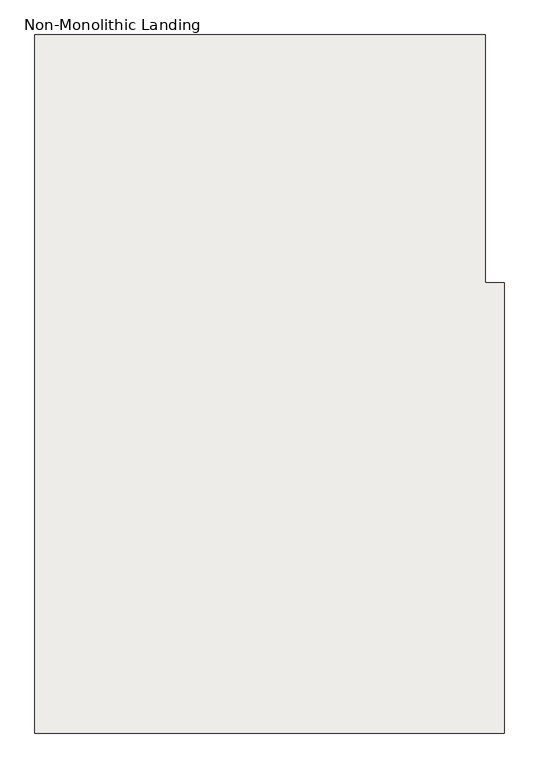
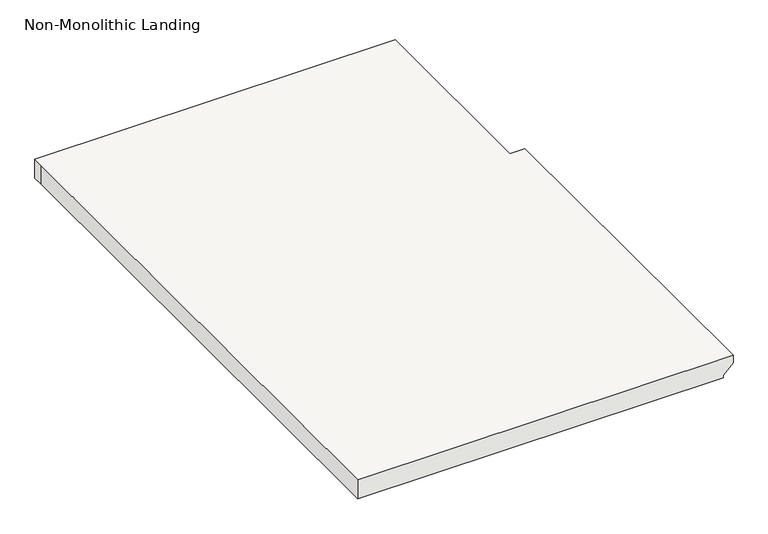
"""IFC4 building model written with IfcOpenShell, lengths in millimetres: slab geometry, Non-Monolithic Landing."""

from ifc_helpers import new_model, si_unit, origin, place, context, project, spatial, faceted_brep, source, transform, mapped, element, save


def non_monolithic_landing_e724ba9d(model_context):
    return source(origin(), model_context, "Body", "Brep", [
        faceted_brep([(-4998.8601025, -2869.057314, 1471.0833333), (-4998.8601025, -2869.057314, 1490.1333333), (-4998.8601025, -3783.457314, 1490.1333333), (-4998.8601025, -3783.457314, 1471.0833333), (-5024.2601025, -2869.057314, 1445.6833333), (-5024.2601025, -3783.457314, 1445.6833333), (-5037.1750936, -2869.057314, 1490.1333333), (-5037.1750936, -2391.1272484, 1490.1333333), (-5037.1750936, -2365.7272484, 1490.1333333), (-5951.5750936, -2365.7272484, 1490.1333333), (-5951.5750936, -2391.1272484, 1490.1333333), (-5951.5750936, -3783.457314, 1490.1333333), (-5024.2601025, -2869.057314, 1439.3333333), (-5024.2601025, -3783.457314, 1439.3333333), (-5951.5750936, -3783.457314, 1439.3333333), (-5951.5750936, -2391.1272484, 1439.3333333), (-5951.5750936, -2365.7272484, 1439.3333333), (-5037.1750936, -2365.7272484, 1439.3333333), (-5037.1750936, -2391.1272484, 1439.3333333), (-5037.1750936, -2869.057314, 1439.3333333)], [[[0, 1, 2, 3]], [[4, 0, 3, 5]], [[6, 7, 8, 9, 10, 11, 2, 1]], [[12, 13, 14, 15, 16, 17, 18, 19]], [[13, 12, 4, 5]], [[6, 1, 0, 4, 12, 19]], [[7, 6, 19, 18]], [[8, 7, 18, 17]], [[9, 8, 17, 16]], [[10, 9, 16, 15]], [[11, 10, 15, 14]], [[2, 11, 14, 13, 5, 3]]]),
    ])


if __name__ == "__main__":
    model = new_model("IFC4")
    model_context = context("Model", 3, world=origin())
    ifc_project = project(units=[si_unit("LENGTHUNIT", "METRE", prefix="MILLI")], contexts=[model_context])
    site = spatial("IfcSite", under=ifc_project)
    building = spatial("IfcBuilding", under=site)
    placement = place(None, origin())
    non_monolithic_landing_shape = non_monolithic_landing_e724ba9d(model_context)
    element("IfcSlab", 1, ObjectType="Non-Monolithic Landing", at=placement, inside=building, context=model_context, shape_type="MappedRepresentation", body=[
        mapped(non_monolithic_landing_shape, transform((0.0, 0.0, 0.0), x_axis=(1.0, 0.0, 0.0), y_axis=(0.0, 1.0, 0.0), z_axis=(0.0, 0.0, 1.0))),
    ])
    save(model, "model.ifc")
